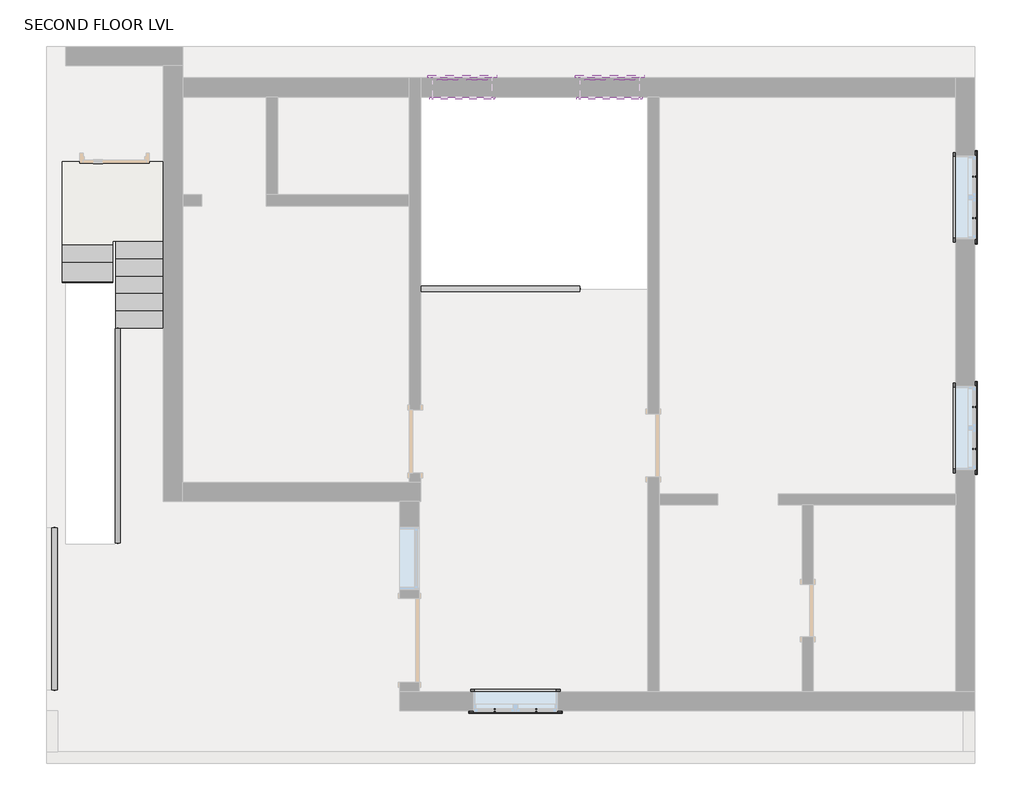
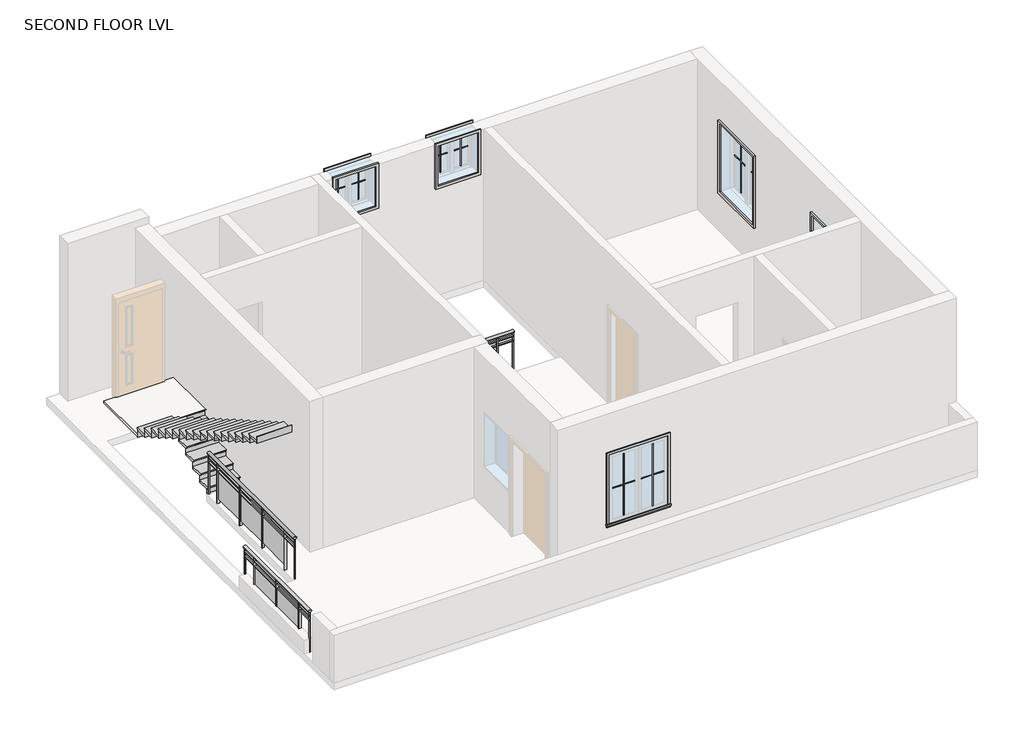
# One storey, part 2 of 2: 20 proxies, 3 railings, 2 stair flights, 1 slab.
"""IFC4 building model written with IfcOpenShell, lengths in millimetres."""

from ifc_helpers import new_model, si_unit, point, frame, origin, place, context, project, spatial, polyline, ellipse_curve, trimmed, outline, extrude, transform, mapped, element, save
from ifc_brep_helpers import plane_surface, extruded_surface, advanced_brep
from components import muntin_pattern_2x2_muntin_pattern_2x2_6dad3731, muntin_pattern_2x2_muntin_pattern_2x2_a30a3345, muntin_pattern_2x2_muntin_pattern_2x2_b3fe6957, muntin_pattern_2x2_muntin_pattern_2x2_3e0ecaf2, trim_window_exterior_flat_with_sill_92b9b949, trim_window_exterior_flat_with_sill_41619996, trim_window_interior_flat_picture_frame_3bb882cf, trim_window_interior_flat_picture_frame_51c85655, non_monolithic_landing_20a8ff8f, stair_flight_670a0b79, stair_flight_246ebb71

model = new_model("IFC4")

# Units and contexts
model_context = context("Model", 3, world=origin())
ifc_project = project(units=[si_unit("LENGTHUNIT", "METRE", prefix="MILLI")], contexts=[model_context])

# Site, building, storey
site = spatial("IfcSite", under=ifc_project)
building = spatial("IfcBuilding", under=site)
storey = spatial("IfcBuildingStorey", under=building, Name="SECOND FLOOR LVL", Elevation=7010.4)

# Proxies
placement = place(None, origin())
muntin_pattern_2x2_muntin_pattern_2x2_shape = muntin_pattern_2x2_muntin_pattern_2x2_6dad3731(model_context)
element("IfcBuildingElementProxy", 1, Name="Muntin Pattern_2x2 : Muntin Pattern_2x2", ObjectType="Muntin Pattern_2x2 : Muntin Pattern_2x2", at=placement, inside=storey, context=model_context, shape_type="MappedRepresentation", body=[
    mapped(muntin_pattern_2x2_muntin_pattern_2x2_shape, transform((46.3469404, -752.1673147, 7994.65), x_axis=(-1.0, 0.0, 0.0), y_axis=(0.0, -1.0, 0.0), z_axis=(0.0, 0.0, 1.0))),
])
element("IfcBuildingElementProxy", 2, Name="Muntin Pattern_2x2 : Muntin Pattern_2x2", ObjectType="Muntin Pattern_2x2 : Muntin Pattern_2x2", at=placement, inside=storey, context=model_context, shape_type="MappedRepresentation", body=[
    mapped(muntin_pattern_2x2_muntin_pattern_2x2_shape, transform((6420.1594404, 3662.6701853, 7994.65), x_axis=(0.0, -1.0, 0.0), y_axis=(1.0, 0.0, 0.0), z_axis=(0.0, 0.0, 1.0))),
])
element("IfcBuildingElementProxy", 3, Name="Muntin Pattern_2x2 : Muntin Pattern_2x2", ObjectType="Muntin Pattern_2x2 : Muntin Pattern_2x2", at=placement, inside=storey, context=model_context, shape_type="MappedRepresentation", body=[
    mapped(muntin_pattern_2x2_muntin_pattern_2x2_shape, transform((6420.1594404, 7021.8201853, 7994.65), x_axis=(0.0, -1.0, 0.0), y_axis=(1.0, 0.0, 0.0), z_axis=(0.0, 0.0, 1.0))),
])
muntin_pattern_2x2_muntin_pattern_2x2_2_shape = muntin_pattern_2x2_muntin_pattern_2x2_a30a3345(model_context)
element("IfcBuildingElementProxy", 4, Name="Muntin Pattern_2x2 : Muntin Pattern_2x2", ObjectType="Muntin Pattern_2x2 : Muntin Pattern_2x2", at=placement, inside=storey, context=model_context, shape_type="MappedRepresentation", body=[
    mapped(muntin_pattern_2x2_muntin_pattern_2x2_2_shape, transform((-560.0780596, -752.1673147, 7994.65), x_axis=(1.0, 0.0, 0.0), y_axis=(0.0, 1.0, 0.0), z_axis=(0.0, 0.0, 1.0))),
])
element("IfcBuildingElementProxy", 5, Name="Muntin Pattern_2x2 : Muntin Pattern_2x2", ObjectType="Muntin Pattern_2x2 : Muntin Pattern_2x2", at=placement, inside=storey, context=model_context, shape_type="MappedRepresentation", body=[
    mapped(muntin_pattern_2x2_muntin_pattern_2x2_2_shape, transform((6420.1594404, 3056.2451853, 7994.65), x_axis=(0.0, 1.0, 0.0), y_axis=(-1.0, 0.0, 0.0), z_axis=(0.0, 0.0, 1.0))),
])
element("IfcBuildingElementProxy", 6, Name="Muntin Pattern_2x2 : Muntin Pattern_2x2", ObjectType="Muntin Pattern_2x2 : Muntin Pattern_2x2", at=placement, inside=storey, context=model_context, shape_type="MappedRepresentation", body=[
    mapped(muntin_pattern_2x2_muntin_pattern_2x2_2_shape, transform((6420.1594404, 6415.3951853, 7994.65), x_axis=(0.0, 1.0, 0.0), y_axis=(-1.0, 0.0, 0.0), z_axis=(0.0, 0.0, 1.0))),
])
muntin_pattern_2x2_muntin_pattern_2x2_3_shape = muntin_pattern_2x2_muntin_pattern_2x2_b3fe6957(model_context)
element("IfcBuildingElementProxy", 7, Name="Muntin Pattern_2x2 : Muntin Pattern_2x2", ObjectType="Muntin Pattern_2x2 : Muntin Pattern_2x2", at=placement, inside=storey, context=model_context, shape_type="MappedRepresentation", body=[
    mapped(muntin_pattern_2x2_muntin_pattern_2x2_3_shape, transform((-1245.8780596, 8448.9826853, 9518.65), x_axis=(1.0, 0.0, 0.0), y_axis=(0.0, 1.0, 0.0), z_axis=(0.0, 0.0, 1.0))),
])
element("IfcBuildingElementProxy", 8, Name="Muntin Pattern_2x2 : Muntin Pattern_2x2", ObjectType="Muntin Pattern_2x2 : Muntin Pattern_2x2", at=placement, inside=storey, context=model_context, shape_type="MappedRepresentation", body=[
    mapped(muntin_pattern_2x2_muntin_pattern_2x2_3_shape, transform((900.4219404, 8448.9826853, 9518.65), x_axis=(1.0, 0.0, 0.0), y_axis=(0.0, 1.0, 0.0), z_axis=(0.0, 0.0, 1.0))),
])
muntin_pattern_2x2_muntin_pattern_2x2_4_shape = muntin_pattern_2x2_muntin_pattern_2x2_3e0ecaf2(model_context)
element("IfcBuildingElementProxy", 9, Name="Muntin Pattern_2x2 : Muntin Pattern_2x2", ObjectType="Muntin Pattern_2x2 : Muntin Pattern_2x2", at=placement, inside=storey, context=model_context, shape_type="MappedRepresentation", body=[
    mapped(muntin_pattern_2x2_muntin_pattern_2x2_4_shape, transform((-817.2530596, 8448.9826853, 9518.65), x_axis=(-1.0, 0.0, 0.0), y_axis=(0.0, -1.0, 0.0), z_axis=(0.0, 0.0, 1.0))),
])
element("IfcBuildingElementProxy", 10, Name="Muntin Pattern_2x2 : Muntin Pattern_2x2", ObjectType="Muntin Pattern_2x2 : Muntin Pattern_2x2", at=placement, inside=storey, context=model_context, shape_type="MappedRepresentation", body=[
    mapped(muntin_pattern_2x2_muntin_pattern_2x2_4_shape, transform((1329.0469404, 8448.9826853, 9518.65), x_axis=(-1.0, 0.0, 0.0), y_axis=(0.0, -1.0, 0.0), z_axis=(0.0, 0.0, 1.0))),
])
trim_window_exterior_flat_with_sill_shape = trim_window_exterior_flat_with_sill_92b9b949(model_context)
element("IfcBuildingElementProxy", 11, Name="Trim-Window-Exterior-Flat : with Sill", ObjectType="Trim-Window-Exterior-Flat : with Sill", at=placement, inside=storey, context=model_context, shape_type="MappedRepresentation", body=[
    mapped(trim_window_exterior_flat_with_sill_shape, transform((-256.8655596, -761.6923147, 9448.8), x_axis=(1.0, 0.0, 0.0), y_axis=(0.0, 0.0, 1.0), z_axis=(0.0, -1.0, 0.0))),
])
element("IfcBuildingElementProxy", 12, Name="Trim-Window-Exterior-Flat : with Sill", ObjectType="Trim-Window-Exterior-Flat : with Sill", at=placement, inside=storey, context=model_context, shape_type="MappedRepresentation", body=[
    mapped(trim_window_exterior_flat_with_sill_shape, transform((6429.6844404, 3359.4576853, 9448.8), x_axis=(0.0, 1.0, 0.0), y_axis=(0.0, 0.0, 1.0), z_axis=(1.0, 0.0, 0.0))),
])
element("IfcBuildingElementProxy", 13, Name="Trim-Window-Exterior-Flat : with Sill", ObjectType="Trim-Window-Exterior-Flat : with Sill", at=placement, inside=storey, context=model_context, shape_type="MappedRepresentation", body=[
    mapped(trim_window_exterior_flat_with_sill_shape, transform((6429.6844404, 6718.6076853, 9448.8), x_axis=(0.0, 1.0, 0.0), y_axis=(0.0, 0.0, 1.0), z_axis=(1.0, 0.0, 0.0))),
])
trim_window_exterior_flat_with_sill_2_shape = trim_window_exterior_flat_with_sill_41619996(model_context)
element("IfcBuildingElementProxy", 14, Name="Trim-Window-Exterior-Flat : with Sill", ObjectType="Trim-Window-Exterior-Flat : with Sill", at=placement, inside=storey, context=model_context, shape_type="MappedRepresentation", body=[
    mapped(trim_window_exterior_flat_with_sill_2_shape, transform((-1031.5655596, 8458.5076853, 10363.2), x_axis=(-1.0, 0.0, 0.0), y_axis=(0.0, 0.0, 1.0), z_axis=(0.0, 1.0, 0.0))),
])
element("IfcBuildingElementProxy", 15, Name="Trim-Window-Exterior-Flat : with Sill", ObjectType="Trim-Window-Exterior-Flat : with Sill", at=placement, inside=storey, context=model_context, shape_type="MappedRepresentation", body=[
    mapped(trim_window_exterior_flat_with_sill_2_shape, transform((1114.7344404, 8458.5076853, 10363.2), x_axis=(-1.0, 0.0, 0.0), y_axis=(0.0, 0.0, 1.0), z_axis=(0.0, 1.0, 0.0))),
])
trim_window_interior_flat_picture_frame_shape = trim_window_interior_flat_picture_frame_3bb882cf(model_context)
element("IfcBuildingElementProxy", 16, Name="Trim-Window-Interior-Flat : Picture Frame", ObjectType="Trim-Window-Interior-Flat : Picture Frame", at=placement, inside=storey, context=model_context, shape_type="MappedRepresentation", body=[
    mapped(trim_window_interior_flat_picture_frame_shape, transform((-256.8655596, -482.2923147, 9448.8), x_axis=(-1.0, 0.0, 0.0), y_axis=(0.0, 0.0, 1.0), z_axis=(0.0, 1.0, 0.0))),
])
element("IfcBuildingElementProxy", 17, Name="Trim-Window-Interior-Flat : Picture Frame", ObjectType="Trim-Window-Interior-Flat : Picture Frame", at=placement, inside=storey, context=model_context, shape_type="MappedRepresentation", body=[
    mapped(trim_window_interior_flat_picture_frame_shape, transform((6150.2844404, 3359.4576853, 9448.8), x_axis=(0.0, -1.0, 0.0), y_axis=(0.0, 0.0, 1.0), z_axis=(-1.0, 0.0, 0.0))),
])
element("IfcBuildingElementProxy", 18, Name="Trim-Window-Interior-Flat : Picture Frame", ObjectType="Trim-Window-Interior-Flat : Picture Frame", at=placement, inside=storey, context=model_context, shape_type="MappedRepresentation", body=[
    mapped(trim_window_interior_flat_picture_frame_shape, transform((6150.2844404, 6718.6076853, 9448.8), x_axis=(0.0, -1.0, 0.0), y_axis=(0.0, 0.0, 1.0), z_axis=(-1.0, 0.0, 0.0))),
])
trim_window_interior_flat_picture_frame_2_shape = trim_window_interior_flat_picture_frame_51c85655(model_context)
element("IfcBuildingElementProxy", 19, Name="Trim-Window-Interior-Flat : Picture Frame", ObjectType="Trim-Window-Interior-Flat : Picture Frame", at=placement, inside=storey, context=model_context, shape_type="MappedRepresentation", body=[
    mapped(trim_window_interior_flat_picture_frame_2_shape, transform((-1031.5655596, 8179.1076853, 10363.2), x_axis=(1.0, 0.0, 0.0), y_axis=(0.0, 0.0, 1.0), z_axis=(0.0, -1.0, 0.0))),
])
element("IfcBuildingElementProxy", 20, Name="Trim-Window-Interior-Flat : Picture Frame", ObjectType="Trim-Window-Interior-Flat : Picture Frame", at=placement, inside=storey, context=model_context, shape_type="MappedRepresentation", body=[
    mapped(trim_window_interior_flat_picture_frame_2_shape, transform((1114.7344404, 8179.1076853, 10363.2), x_axis=(1.0, 0.0, 0.0), y_axis=(0.0, 0.0, 1.0), z_axis=(0.0, -1.0, 0.0))),
])

# Railings
element("IfcRailing", 21, ObjectType="Glass Panel - Bottom Fill", at=placement, inside=storey, context=model_context, shape_type="SolidModel", body=[
    advanced_brep(
    [(676.5844404, 5347.0076853, 7924.8), (676.5844404, 5423.2076853, 7924.8), (-1634.8155596, 5347.0076853, 7924.8), (-1634.8155596, 5423.2076853, 7924.8)],
    [
        (0, 1, ellipse_curve(frame((676.5844404, 5385.1076853, 7924.8), z_axis=(1.0, 0.0, 0.0), x_axis=(0.0, 1.0, 0.0)), 38.1, 28.575)),
        (1, 0, ellipse_curve(frame((676.5844404, 5385.1076853, 7924.8), z_axis=(1.0, 0.0, 0.0), x_axis=(0.0, 1.0, 0.0)), 38.1, 28.575)),
        (2, 3, ellipse_curve(frame((-1634.8155596, 5385.1076853, 7924.8), z_axis=(-1.0, 0.0, 0.0), x_axis=(0.0, 1.0, 0.0)), 38.1, 28.575)),
        (3, 2, ellipse_curve(frame((-1634.8155596, 5385.1076853, 7924.8), z_axis=(-1.0, 0.0, 0.0), x_axis=(0.0, 1.0, 0.0)), 38.1, 28.575)),
        (0, 2),
        (3, 1),
    ],
    [
        plane_surface(frame((676.5844404, 5385.1076853, 7924.8), z_axis=(1.0, 0.0, 0.0), x_axis=(0.0, -1.0, 0.0))),
        plane_surface(frame((-1634.8155596, 5385.1076853, 7924.8), z_axis=(-1.0, 0.0, 0.0), x_axis=(0.0, -1.0, 0.0))),
        extruded_surface(trimmed(ellipse_curve(frame((-1634.8155596, 5385.1076853, 7924.8), z_axis=(1.0, 0.0, 0.0), x_axis=(0.0, 1.0, 0.0)), 38.1, 28.575), [point((-1634.8155596, 5347.0076853, 7924.8))], [point((-1634.8155596, 5423.2076853, 7924.8))], True, "CARTESIAN"), (2311.3999999999996, 0.0, 0.0), 2311.3999999999996),
        extruded_surface(trimmed(ellipse_curve(frame((-1634.8155596, 5385.1076853, 7924.8), z_axis=(1.0, 0.0, 0.0), x_axis=(0.0, 1.0, 0.0)), 38.1, 28.575), [point((-1634.8155596, 5423.2076853, 7924.8))], [point((-1634.8155596, 5347.0076853, 7924.8))], True, "CARTESIAN"), (2311.3999999999996, 0.0, 0.0), 2311.3999999999996),
    ],
    [
        (0, [[1, 2]]),
        (1, [[3, 4]]),
        (2, [[-1, 5, -4, 6]]),
        (3, [[-2, -6, -3, -5]]),
    ],
),
    extrude(outline(polyline([(676.5844404, 5397.8076853), (676.5844404, 5372.4076853), (-1634.8155596, 5372.4076853), (-1634.8155596, 5397.8076853), (676.5844404, 5397.8076853)])), frame((0.0, 0.0, 7810.5), z_axis=(0.0, 0.0, 1.0), x_axis=(1.0, 0.0, 0.0)), (0.0, 0.0, 1.0), 25.4),
    extrude(outline(polyline([(676.5844404, 5397.8076853), (676.5844404, 5372.4076853), (-1634.8155596, 5372.4076853), (-1634.8155596, 5397.8076853), (676.5844404, 5397.8076853)])), frame((0.0, 0.0, 7708.9), z_axis=(0.0, 0.0, 1.0), x_axis=(1.0, 0.0, 0.0)), (0.0, 0.0, 1.0), 25.4),
    extrude(outline(polyline([(-1285.5655596, 5359.7076853), (-1298.2655596, 5359.7076853), (-1298.2655596, 5410.5076853), (-1285.5655596, 5410.5076853), (-1285.5655596, 5359.7076853)])), frame((0.0, 0.0, 7010.4), z_axis=(0.0, 0.0, 1.0), x_axis=(1.0, 0.0, 0.0)), (0.0, 0.0, 1.0), 885.825),
    extrude(outline(polyline([(-479.1155596, 5391.6428423), (-479.1155596, 5385.2928423), (-1291.9155596, 5385.2928423), (-1291.9155596, 5391.6428423), (-479.1155596, 5391.6428423)])), frame((0.0, 0.0, 7112.0), z_axis=(0.0, 0.0, 1.0), x_axis=(1.0, 0.0, 0.0)), (0.0, 0.0, 1.0), 596.9),
    extrude(outline(polyline([(-472.7655596, 5359.7076853), (-485.4655596, 5359.7076853), (-485.4655596, 5410.5076853), (-472.7655596, 5410.5076853), (-472.7655596, 5359.7076853)])), frame((0.0, 0.0, 7010.4), z_axis=(0.0, 0.0, 1.0), x_axis=(1.0, 0.0, 0.0)), (0.0, 0.0, 1.0), 885.825),
    extrude(outline(polyline([(333.6844404, 5391.6428423), (333.6844404, 5385.2928423), (-479.1155596, 5385.2928423), (-479.1155596, 5391.6428423), (333.6844404, 5391.6428423)])), frame((0.0, 0.0, 7112.0), z_axis=(0.0, 0.0, 1.0), x_axis=(1.0, 0.0, 0.0)), (0.0, 0.0, 1.0), 596.9),
    extrude(outline(polyline([(340.0344404, 5359.7076853), (327.3344404, 5359.7076853), (327.3344404, 5410.5076853), (340.0344404, 5410.5076853), (340.0344404, 5359.7076853)])), frame((0.0, 0.0, 7010.4), z_axis=(0.0, 0.0, 1.0), x_axis=(1.0, 0.0, 0.0)), (0.0, 0.0, 1.0), 885.825),
    extrude(outline(polyline([(-1622.1155596, 5375.5826853), (-1641.1655596, 5375.5826853), (-1641.1655596, 5394.6326853), (-1622.1155596, 5394.6326853), (-1622.1155596, 5375.5826853)])), frame((0.0, 0.0, 7010.4), z_axis=(0.0, 0.0, 1.0), x_axis=(1.0, 0.0, 0.0)), (0.0, 0.0, 1.0), 885.825),
    extrude(outline(polyline([(682.9344404, 5375.5826853), (663.8844404, 5375.5826853), (663.8844404, 5394.6326853), (682.9344404, 5394.6326853), (682.9344404, 5375.5826853)])), frame((0.0, 0.0, 7010.4), z_axis=(0.0, 0.0, 1.0), x_axis=(1.0, 0.0, 0.0)), (0.0, 0.0, 1.0), 885.825),
])
element("IfcRailing", 22, ObjectType="Glass Panel - Bottom Fill", at=placement, inside=storey, context=model_context, shape_type="SolidModel", body=[
    advanced_brep(
    [(-6008.6955596, 4807.2576853, 7924.8), (-6084.8955596, 4807.2576853, 7924.8), (-6008.6955596, 1683.0576853, 7924.8), (-6084.8955596, 1683.0576853, 7924.8)],
    [
        (0, 1, ellipse_curve(frame((-6046.7955596, 4807.2576853, 7924.8), z_axis=(0.0, 1.0, 0.0), x_axis=(-1.0, 0.0, 0.0)), 38.1, 28.575)),
        (1, 0, ellipse_curve(frame((-6046.7955596, 4807.2576853, 7924.8), z_axis=(0.0, 1.0, 0.0), x_axis=(-1.0, 0.0, 0.0)), 38.1, 28.575)),
        (2, 3, ellipse_curve(frame((-6046.7955596, 1683.0576853, 7924.8), z_axis=(0.0, -1.0, 0.0), x_axis=(-1.0, 0.0, 0.0)), 38.1, 28.575)),
        (3, 2, ellipse_curve(frame((-6046.7955596, 1683.0576853, 7924.8), z_axis=(0.0, -1.0, 0.0), x_axis=(-1.0, 0.0, 0.0)), 38.1, 28.575)),
        (0, 2),
        (3, 1),
    ],
    [
        plane_surface(frame((-6046.7955596, 4807.2576853, 7924.8), z_axis=(0.0, 1.0, 0.0), x_axis=(0.0, 0.0, -1.0))),
        plane_surface(frame((-6046.7955596, 1683.0576853, 7924.8), z_axis=(0.0, -1.0, 0.0), x_axis=(0.0, 0.0, -1.0))),
        extruded_surface(trimmed(ellipse_curve(frame((-6046.7955596, 1683.0576853, 7924.8), z_axis=(0.0, 1.0, 0.0), x_axis=(-1.0, 0.0, 0.0)), 38.1, 28.575), [point((-6008.6955596, 1683.0576853, 7924.8))], [point((-6084.8955596, 1683.0576853, 7924.8))], True, "CARTESIAN"), (0.0, 3124.2, 0.0), 3124.2),
        extruded_surface(trimmed(ellipse_curve(frame((-6046.7955596, 1683.0576853, 7924.8), z_axis=(0.0, 1.0, 0.0), x_axis=(-1.0, 0.0, 0.0)), 38.1, 28.575), [point((-6084.8955596, 1683.0576853, 7924.8))], [point((-6008.6955596, 1683.0576853, 7924.8))], True, "CARTESIAN"), (0.0, 3124.2, 0.0), 3124.2),
    ],
    [
        (0, [[1, 2]]),
        (1, [[3, 4]]),
        (2, [[-1, 5, -4, 6]]),
        (3, [[-2, -6, -3, -5]]),
    ],
),
    extrude(outline(polyline([(-6059.4955596, 4807.2576853), (-6034.0955596, 4807.2576853), (-6034.0955596, 1683.0576853), (-6059.4955596, 1683.0576853), (-6059.4955596, 4807.2576853)])), frame((0.0, 0.0, 7810.5), z_axis=(0.0, 0.0, 1.0), x_axis=(1.0, 0.0, 0.0)), (0.0, 0.0, 1.0), 25.4),
    extrude(outline(polyline([(-6059.4955596, 4807.2576853), (-6034.0955596, 4807.2576853), (-6034.0955596, 1683.0576853), (-6059.4955596, 1683.0576853), (-6059.4955596, 4807.2576853)])), frame((0.0, 0.0, 7708.9), z_axis=(0.0, 0.0, 1.0), x_axis=(1.0, 0.0, 0.0)), (0.0, 0.0, 1.0), 25.4),
    extrude(outline(polyline([(-6072.1955596, 2032.3076853), (-6021.3955596, 2032.3076853), (-6021.3955596, 2019.6076853), (-6072.1955596, 2019.6076853), (-6072.1955596, 2032.3076853)])), frame((0.0, 0.0, 7010.4), z_axis=(0.0, 0.0, 1.0), x_axis=(1.0, 0.0, 0.0)), (0.0, 0.0, 1.0), 885.825),
    extrude(outline(polyline([(-6040.2604026, 2838.7576853), (-6040.2604026, 2025.9576853), (-6046.6104026, 2025.9576853), (-6046.6104026, 2838.7576853), (-6040.2604026, 2838.7576853)])), frame((0.0, 0.0, 7112.0), z_axis=(0.0, 0.0, 1.0), x_axis=(1.0, 0.0, 0.0)), (0.0, 0.0, 1.0), 596.9),
    extrude(outline(polyline([(-6072.1955596, 2845.1076853), (-6021.3955596, 2845.1076853), (-6021.3955596, 2832.4076853), (-6072.1955596, 2832.4076853), (-6072.1955596, 2845.1076853)])), frame((0.0, 0.0, 7010.4), z_axis=(0.0, 0.0, 1.0), x_axis=(1.0, 0.0, 0.0)), (0.0, 0.0, 1.0), 885.825),
    extrude(outline(polyline([(-6040.2604026, 3651.5576853), (-6040.2604026, 2838.7576853), (-6046.6104026, 2838.7576853), (-6046.6104026, 3651.5576853), (-6040.2604026, 3651.5576853)])), frame((0.0, 0.0, 7112.0), z_axis=(0.0, 0.0, 1.0), x_axis=(1.0, 0.0, 0.0)), (0.0, 0.0, 1.0), 596.9),
    extrude(outline(polyline([(-6072.1955596, 3657.9076853), (-6021.3955596, 3657.9076853), (-6021.3955596, 3645.2076853), (-6072.1955596, 3645.2076853), (-6072.1955596, 3657.9076853)])), frame((0.0, 0.0, 7010.4), z_axis=(0.0, 0.0, 1.0), x_axis=(1.0, 0.0, 0.0)), (0.0, 0.0, 1.0), 885.825),
    extrude(outline(polyline([(-6040.2604026, 4464.3576853), (-6040.2604026, 3651.5576853), (-6046.6104026, 3651.5576853), (-6046.6104026, 4464.3576853), (-6040.2604026, 4464.3576853)])), frame((0.0, 0.0, 7112.0), z_axis=(0.0, 0.0, 1.0), x_axis=(1.0, 0.0, 0.0)), (0.0, 0.0, 1.0), 596.9),
    extrude(outline(polyline([(-6072.1955596, 4470.7076853), (-6021.3955596, 4470.7076853), (-6021.3955596, 4458.0076853), (-6072.1955596, 4458.0076853), (-6072.1955596, 4470.7076853)])), frame((0.0, 0.0, 7010.4), z_axis=(0.0, 0.0, 1.0), x_axis=(1.0, 0.0, 0.0)), (0.0, 0.0, 1.0), 885.825),
    extrude(outline(polyline([(-6056.3205596, 1695.7576853), (-6037.2705596, 1695.7576853), (-6037.2705596, 1676.7076853), (-6056.3205596, 1676.7076853), (-6056.3205596, 1695.7576853)])), frame((0.0, 0.0, 7010.4), z_axis=(0.0, 0.0, 1.0), x_axis=(1.0, 0.0, 0.0)), (0.0, 0.0, 1.0), 885.825),
    extrude(outline(polyline([(-6056.3205596, 4813.6076853), (-6037.2705596, 4813.6076853), (-6037.2705596, 4794.5576853), (-6056.3205596, 4794.5576853), (-6056.3205596, 4813.6076853)])), frame((0.0, 0.0, 7010.4), z_axis=(0.0, 0.0, 1.0), x_axis=(1.0, 0.0, 0.0)), (0.0, 0.0, 1.0), 885.825),
])
element("IfcRailing", 23, ObjectType="Glass Panel - Bottom Fill", at=placement, inside=storey, context=model_context, shape_type="SolidModel", body=[
    advanced_brep(
    [(-7006.9155596, -456.8923147, 7924.8), (-6930.7155596, -456.8923147, 7924.8), (-7006.9155596, 1905.3076853, 7924.8), (-6930.7155596, 1905.3076853, 7924.8)],
    [
        (0, 1, ellipse_curve(frame((-6968.8155596, -456.8923147, 7924.8), z_axis=(0.0, -1.0, 0.0), x_axis=(1.0, 0.0, 0.0)), 38.1, 28.575)),
        (1, 0, ellipse_curve(frame((-6968.8155596, -456.8923147, 7924.8), z_axis=(0.0, -1.0, 0.0), x_axis=(1.0, 0.0, 0.0)), 38.1, 28.575)),
        (2, 3, ellipse_curve(frame((-6968.8155596, 1905.3076853, 7924.8), z_axis=(0.0, 1.0, 0.0), x_axis=(1.0, 0.0, 0.0)), 38.1, 28.575)),
        (3, 2, ellipse_curve(frame((-6968.8155596, 1905.3076853, 7924.8), z_axis=(0.0, 1.0, 0.0), x_axis=(1.0, 0.0, 0.0)), 38.1, 28.575)),
        (0, 2),
        (3, 1),
    ],
    [
        plane_surface(frame((-6968.8155596, -456.8923147, 7924.8), z_axis=(0.0, -1.0, 0.0), x_axis=(0.0, 0.0, 1.0))),
        plane_surface(frame((-6968.8155596, 1905.3076853, 7924.8), z_axis=(0.0, 1.0, 0.0), x_axis=(0.0, 0.0, 1.0))),
        extruded_surface(trimmed(ellipse_curve(frame((-6968.8155596, 1905.3076853, 7924.8), z_axis=(0.0, -1.0, 0.0), x_axis=(1.0, 0.0, 0.0)), 38.1, 28.575), [point((-7006.9155596, 1905.3076853, 7924.8))], [point((-6930.7155596, 1905.3076853, 7924.8))], True, "CARTESIAN"), (0.0, -2362.2, 0.0), 2362.2),
        extruded_surface(trimmed(ellipse_curve(frame((-6968.8155596, 1905.3076853, 7924.8), z_axis=(0.0, -1.0, 0.0), x_axis=(1.0, 0.0, 0.0)), 38.1, 28.575), [point((-6930.7155596, 1905.3076853, 7924.8))], [point((-7006.9155596, 1905.3076853, 7924.8))], True, "CARTESIAN"), (0.0, -2362.2, 0.0), 2362.2),
    ],
    [
        (0, [[1, 2]]),
        (1, [[3, 4]]),
        (2, [[-1, 5, -4, 6]]),
        (3, [[-2, -6, -3, -5]]),
    ],
),
    extrude(outline(polyline([(-6956.1155596, -456.8923147), (-6981.5155596, -456.8923147), (-6981.5155596, 1905.3076853), (-6956.1155596, 1905.3076853), (-6956.1155596, -456.8923147)])), frame((0.0, 0.0, 7810.5), z_axis=(0.0, 0.0, 1.0), x_axis=(1.0, 0.0, 0.0)), (0.0, 0.0, 1.0), 25.4),
    extrude(outline(polyline([(-6956.1155596, -456.8923147), (-6981.5155596, -456.8923147), (-6981.5155596, 1905.3076853), (-6956.1155596, 1905.3076853), (-6956.1155596, -456.8923147)])), frame((0.0, 0.0, 7708.9), z_axis=(0.0, 0.0, 1.0), x_axis=(1.0, 0.0, 0.0)), (0.0, 0.0, 1.0), 25.4),
    extrude(outline(polyline([(-6943.4155596, 1530.6576853), (-6994.2155596, 1530.6576853), (-6994.2155596, 1543.3576853), (-6943.4155596, 1543.3576853), (-6943.4155596, 1530.6576853)])), frame((0.0, 0.0, 7010.4), z_axis=(0.0, 0.0, 1.0), x_axis=(1.0, 0.0, 0.0)), (0.0, 0.0, 1.0), 885.825),
    extrude(outline(polyline([(-6975.3507166, 724.2076853), (-6975.3507166, 1537.0076853), (-6969.0007166, 1537.0076853), (-6969.0007166, 724.2076853), (-6975.3507166, 724.2076853)])), frame((0.0, 0.0, 7112.0), z_axis=(0.0, 0.0, 1.0), x_axis=(1.0, 0.0, 0.0)), (0.0, 0.0, 1.0), 596.9),
    extrude(outline(polyline([(-6943.4155596, 717.8576853), (-6994.2155596, 717.8576853), (-6994.2155596, 730.5576853), (-6943.4155596, 730.5576853), (-6943.4155596, 717.8576853)])), frame((0.0, 0.0, 7010.4), z_axis=(0.0, 0.0, 1.0), x_axis=(1.0, 0.0, 0.0)), (0.0, 0.0, 1.0), 885.825),
    extrude(outline(polyline([(-6975.3507166, -88.5923147), (-6975.3507166, 724.2076853), (-6969.0007166, 724.2076853), (-6969.0007166, -88.5923147), (-6975.3507166, -88.5923147)])), frame((0.0, 0.0, 7112.0), z_axis=(0.0, 0.0, 1.0), x_axis=(1.0, 0.0, 0.0)), (0.0, 0.0, 1.0), 596.9),
    extrude(outline(polyline([(-6943.4155596, -94.9423147), (-6994.2155596, -94.9423147), (-6994.2155596, -82.2423147), (-6943.4155596, -82.2423147), (-6943.4155596, -94.9423147)])), frame((0.0, 0.0, 7010.4), z_axis=(0.0, 0.0, 1.0), x_axis=(1.0, 0.0, 0.0)), (0.0, 0.0, 1.0), 885.825),
    extrude(outline(polyline([(-6959.2905596, 1892.6076853), (-6978.3405596, 1892.6076853), (-6978.3405596, 1911.6576853), (-6959.2905596, 1911.6576853), (-6959.2905596, 1892.6076853)])), frame((0.0, 0.0, 7010.4), z_axis=(0.0, 0.0, 1.0), x_axis=(1.0, 0.0, 0.0)), (0.0, 0.0, 1.0), 885.825),
    extrude(outline(polyline([(-6959.2905596, -463.2423147), (-6978.3405596, -463.2423147), (-6978.3405596, -444.1923147), (-6959.2905596, -444.1923147), (-6959.2905596, -463.2423147)])), frame((0.0, 0.0, 7010.4), z_axis=(0.0, 0.0, 1.0), x_axis=(1.0, 0.0, 0.0)), (0.0, 0.0, 1.0), 885.825),
])

# Slab
non_monolithic_landing_shape = non_monolithic_landing_20a8ff8f(model_context)
element("IfcSlab", 24, ObjectType="Non-Monolithic Landing", at=placement, inside=storey, context=model_context, shape_type="MappedRepresentation", body=[
    mapped(non_monolithic_landing_shape, transform((0.0, 0.0, 0.0), x_axis=(1.0, 0.0, 0.0), y_axis=(0.0, 1.0, 0.0), z_axis=(0.0, 0.0, 1.0))),
])

# Stair flights
stair_flight_shape = stair_flight_670a0b79(model_context)
element("IfcStairFlight", 25, ObjectType="2\" Tread 1\" Nosing 1/4\" Riser", at=placement, inside=storey, context=model_context, shape_type="MappedRepresentation", body=[
    mapped(stair_flight_shape, transform((0.0, 0.0, 0.0), x_axis=(1.0, 0.0, 0.0), y_axis=(0.0, 1.0, 0.0), z_axis=(0.0, 0.0, 1.0))),
])
stair_flight_2_shape = stair_flight_246ebb71(model_context)
element("IfcStairFlight", 26, ObjectType="2\" Tread 1\" Nosing 1/4\" Riser", at=placement, inside=storey, context=model_context, shape_type="MappedRepresentation", body=[
    mapped(stair_flight_2_shape, transform((0.0, 0.0, 0.0), x_axis=(1.0, 0.0, 0.0), y_axis=(0.0, 1.0, 0.0), z_axis=(0.0, 0.0, 1.0))),
])

save(model, "model.ifc")

# Revit data of these elements
# Type "Muntin Pattern_2x2 : Muntin Pattern_2x2"
#   Width [instance default] = 4' - 0"
#   Thickness = 0' - 0 1/2"
#   Height [instance default] = 4' - 0"
#   Distance = 0' - 0 3/4"
#   Interior Material [instance default] = none
#   Exterior Material [instance default] = none
#   Default Elevation = 0
# Type "Trim-Window-Exterior-Flat : with Sill"
#   Trim Width = 0' - 2 1/4"
#   Trim Thickness_Picture Frame = 0' - 1 1/4"
#   Trim Thickness_with Sill = 0' - 0 3/4"
#   Sill Thickness = 0' - 1 1/4"
#   Opening Width [instance default] = 2' - 0"
#   Opening Height [instance default] = 3' - 0"
#   Default Elevation = 4' - 0"
#   Sill = yes
#   Picture Frame = no
#   Trim Material [instance default] = none
# Type "Trim-Window-Interior-Flat : Picture Frame"
#   Trim Thickness_Picture Frame = 0' - 1 1/4"
#   Trim Width = 0' - 2 1/4"
#   Trim Thickness_with Sill = 0' - 0 3/4"
#   Sill Thickness = 0' - 1 1/4"
#   Opening Width [instance default] = 2' - 0"
#   Opening Height [instance default] = 3' - 0"
#   Default Elevation = 4' - 0"
#   Sill = no
#   Picture Frame = yes
#   Trim Material [instance default] = none
# Type "Glass Panel - Bottom Fill"
#   Assembly Code = "C2010400"
#   built-in parameter 1008612 = 0.0416667 (stored number, unit not read)
#   built-in parameter 1008611 = 0.0416667 (stored number, unit not read)
#   built-in parameter 1008609 = 0.333333 (stored number, unit not read)
#   built-in parameter 1008604 = 0.166667 (stored number, unit not read)
#   built-in parameter 1008603 = 0.166667 (stored number, unit not read)
#   Railing Height = 3' - 0"
#   built-in parameter 1008630 = 2
#   built-in parameter 1008610 = 2
#   built-in parameter 1008618 = Baluster - Square : 3/4"
# Elements 1, 2, 3, 4, 5, 6 (IfcBuildingElementProxy, "Muntin Pattern_2x2 : Muntin Pattern_2x2")
#   Width = 1' - 6 5/8"
#   Height = 4' - 6 1/2"
#   Interior Material = Wood - Stained
#   Exterior Material = Clad - White
#   Phase Created = New Construction
#   Materials on its faces: "Clad - White", "Wood - Stained"
# Elements 7, 8, 9, 10 (IfcBuildingElementProxy, "Muntin Pattern_2x2 : Muntin Pattern_2x2")
#   Width = 0' - 11 5/8"
#   Height = 2' - 6 1/2"
#   Interior Material = Wood - Stained
#   Exterior Material = Clad - White
#   Phase Created = New Construction
#   Materials on its faces: "Clad - White", "Wood - Stained"
# Elements 11, 12, 13 (IfcBuildingElementProxy, "Trim-Window-Exterior-Flat : with Sill")
#   Opening Width = 4' - 0"
#   Opening Height = 5' - 0"
#   Trim Material = Clad - White
#   Phase Created = New Construction
#   Materials on its faces: "Clad - White"
# Elements 14, 15 (IfcBuildingElementProxy, "Trim-Window-Exterior-Flat : with Sill")
#   Opening Width = 2' - 10"
#   Opening Height = 3' - 0"
#   Trim Material = Clad - White
#   Phase Created = New Construction
#   Materials on its faces: "Clad - White"
# Elements 16, 17, 18 (IfcBuildingElementProxy, "Trim-Window-Interior-Flat : Picture Frame")
#   Opening Width = 4' - 0"
#   Opening Height = 5' - 0"
#   Trim Material = Wood - Stained
#   Phase Created = New Construction
#   Materials on its faces: "Wood - Stained"
# Elements 19, 20 (IfcBuildingElementProxy, "Trim-Window-Interior-Flat : Picture Frame")
#   Opening Width = 2' - 10"
#   Opening Height = 3' - 0"
#   Trim Material = Wood - Stained
#   Phase Created = New Construction
#   Materials on its faces: "Wood - Stained"
# Elements 21, 22, 23 (IfcRailing, "Glass Panel - Bottom Fill")
#   Phase Created = New Construction
#   Materials on its faces: "Glass"
# Element 24 (IfcSlab, "Non-Monolithic Landing")
#   Phase Created = New Construction
# Elements 25, 26 (IfcStairFlight, "2\" Tread 1\" Nosing 1/4\" Riser")
#   Phase Created = New Construction
# Materials
#   "Clad - White": class "Wood", colour RGB 242 242 238, transparency 0, Cost = 0
#   "Wood - Stained": class "Wood", colour RGB 224 178 126, transparency 0, Cost = 0
#   "Glass": class "Glass", colour RGB 0 128 192, transparency 0.75, Description = "Soda Lime Glass", Cost = 0
